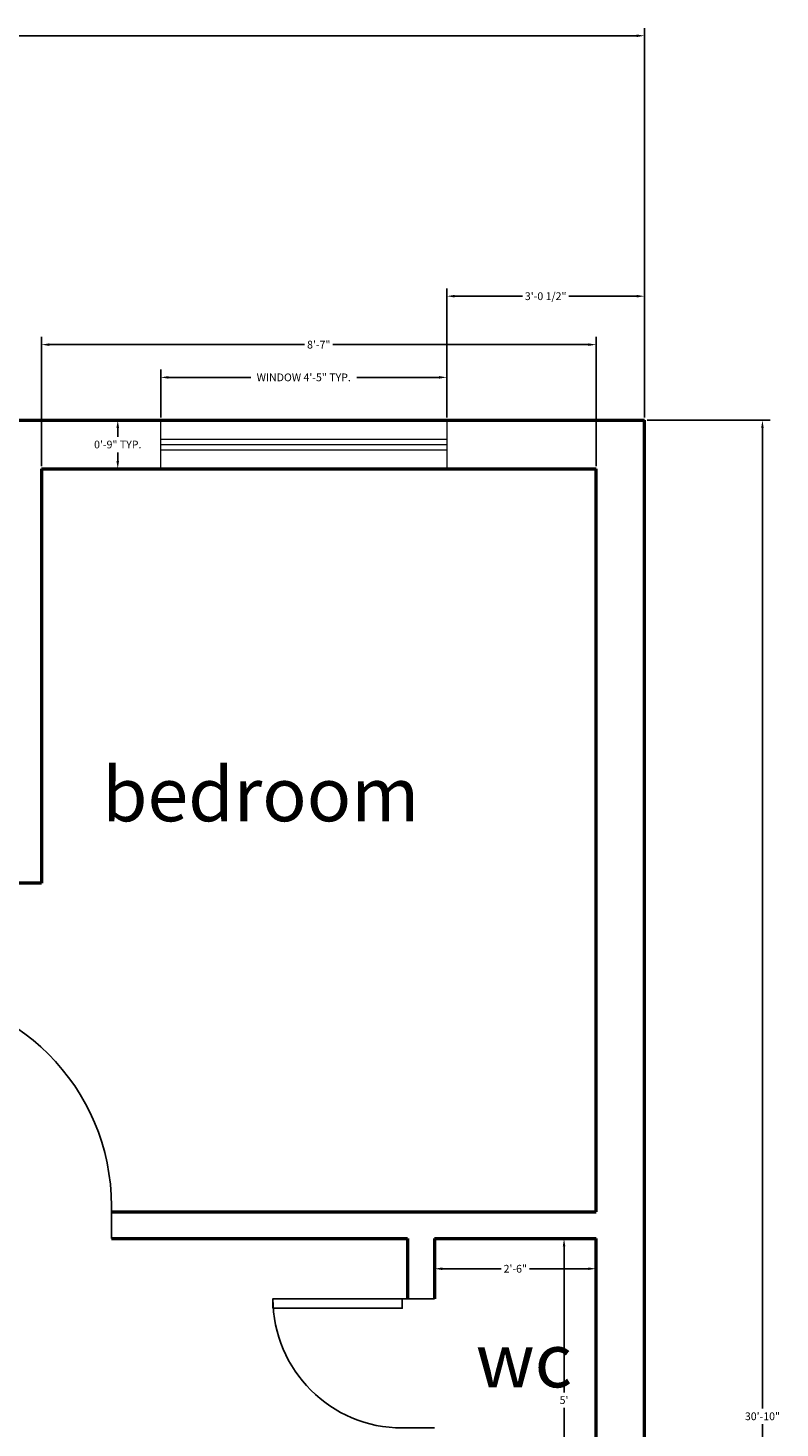
# Model space of a CAD drawing. Units: inches. Extents: x 325 to 804, y 366 to 834.
# Tile 6 of 6: x 660 to 800, y 574 to 834. Entities that reach past the tile are written whole.
import ezdxf

# ---------------------------------------------------------------- set-up
doc = ezdxf.new("R2010")
doc.units = ezdxf.units.IN
doc.header["$MEASUREMENT"] = 0
doc.layers.get('0').update_dxf_attribs({"color": 4})
for name, color, linetype, lineweight in [('A-ANNO-DIMS', 2, 'Continuous', 18), ('A-AREA-IDEN', 7, 'Continuous', 25), ('A-WALL', 7, 'Continuous', 50), ('door', 10, 'Continuous', 25), ('window', 3, 'Continuous', 18)]:
    doc.layers.add(name, color=color, linetype=linetype, lineweight=lineweight)
doc.styles.get("Standard").update_dxf_attribs({"font": 'arial.ttf'})
doc.dimstyles.get("Standard").update_dxf_attribs({"dimscale": 8, "dimtxt": 0.18, "dimasz": 0.18, "dimexe": 0.18, "dimexo": 0.0625, "dimgap": 0.09, "dimtad": 0, "dimtih": 1, "dimtoh": 1, "dimdec": 0, "dimzin": 0, "dimdsep": 46, "dimlunit": 3, "dimtxsty": 'Standard', "dimcen": 0.09, "dimadec": 0, "dimazin": 0, "dimtfac": 1, "dimtdec": 0, "dimtofl": 0, "dimtmove": 0, "dimatfit": 3, "dimfxl": 1, "dimtolj": 1, "dimtzin": 0, "dimarcsym": 0})

# ---------------------------------------------------------------- blocks, each defined once
blk = doc.blocks.new('*U2')
for p, q in [((0, 0), (0, -6)), ((-40, 0), (-40, -6))]:
    blk.add_line(p, q)
blk.add_lwpolyline([(0, 0), (0, 40), (-1.75, 40), (-1.75, 0)], close=True)
blk.add_arc((0, 0), 40, 90, 180)
blk = doc.blocks.new('*U8')
for p, q in [((-24, 0), (-24, -6)), ((0, 0), (0, -6))]:
    blk.add_line(p, q)
blk.add_lwpolyline([(0, 0), (0, 24), (-1.75, 24), (-1.75, 0)], close=True)
blk.add_arc((0, 0), 24, 90, 180)
blk = doc.blocks.new('*D21')
at = {"layer": 'A-ANNO-DIMS', "color": 0, "lineweight": -2, "transparency": 16777216}
for p, q in [((764.97, 609.54), (758.08, 609.54)), ((759.52, 608.1), (759.52, 580.99)), ((759.52, 550.98), (759.52, 578.09)), ((764.97, 549.54), (758.08, 549.54))]:
    blk.add_line(p, q, dxfattribs=at)
at = {"layer": 'A-ANNO-DIMS', "color": 0, "transparency": 16777216}
for points in [[(759.28, 608.1), (759.76, 608.1), (759.52, 609.54)], [(759.28, 550.98), (759.76, 550.98), (759.52, 549.54)]]:
    blk.add_solid(points, dxfattribs=at)
at = {"layer": 'Defpoints', "color": 0, "transparency": 16777216}
for p in [(765.47, 609.54), (759.52, 549.54), (765.47, 549.54)]:
    blk.add_point(p, dxfattribs=at)
at = {"layer": 'A-ANNO-DIMS', "color": 0, "transparency": 16777216, "insert": (759.52, 579.54), "char_height": 1.44, "attachment_point": 5}
blk.add_mtext("\\A1;5'", dxfattribs=at)
blk = doc.blocks.new('*D22')
at = {"layer": 'A-ANNO-DIMS', "color": 0, "lineweight": -2, "transparency": 16777216}
for p, q in [((735.47, 609.04), (735.47, 602.51)), ((765.47, 609.04), (765.47, 602.51)), ((736.91, 603.95), (747.83, 603.95)), ((764.03, 603.95), (753.12, 603.95))]:
    blk.add_line(p, q, dxfattribs=at)
at = {"layer": 'A-ANNO-DIMS', "color": 0, "transparency": 16777216}
for points in [[(736.91, 604.19), (736.91, 603.71), (735.47, 603.95)], [(764.03, 604.19), (764.03, 603.71), (765.47, 603.95)]]:
    blk.add_solid(points, dxfattribs=at)
at = {"layer": 'Defpoints', "color": 0, "transparency": 16777216}
for p in [(735.47, 609.54), (765.47, 609.54), (735.47, 603.95)]:
    blk.add_point(p, dxfattribs=at)
at = {"layer": 'A-ANNO-DIMS', "color": 0, "transparency": 16777216, "insert": (750.47, 603.95), "char_height": 1.44, "attachment_point": 5}
blk.add_mtext('\\A1;2\'-6"', dxfattribs=at)
blk = doc.blocks.new('*D25')
at = {"layer": 'A-ANNO-DIMS', "color": 0, "lineweight": -2, "transparency": 16777216}
for p, q in [((350.47, 762.04), (350.47, 834.4)), ((351.91, 832.96), (559.28, 832.96)), ((773.03, 832.96), (565.67, 832.96)), ((774.47, 762.04), (774.47, 834.4))]:
    blk.add_line(p, q, dxfattribs=at)
at = {"layer": 'A-ANNO-DIMS', "color": 0, "transparency": 16777216}
for points in [[(351.91, 833.2), (351.91, 832.72), (350.47, 832.96)], [(773.03, 833.2), (773.03, 832.72), (774.47, 832.96)]]:
    blk.add_solid(points, dxfattribs=at)
at = {"layer": 'Defpoints', "color": 0, "transparency": 16777216}
for p in [(774.47, 832.96), (350.47, 761.54), (774.47, 761.54)]:
    blk.add_point(p, dxfattribs=at)
at = {"layer": 'A-ANNO-DIMS', "color": 0, "transparency": 16777216, "insert": (562.47, 832.96), "char_height": 1.44, "attachment_point": 5}
blk.add_mtext('\\A1;35\'-4"', dxfattribs=at)
blk = doc.blocks.new('*D26')
at = {"layer": 'A-ANNO-DIMS', "color": 0, "lineweight": -2, "transparency": 16777216}
for p, q in [((774.97, 761.54), (797.81, 761.54)), ((796.37, 760.1), (796.37, 577.99)), ((796.37, 392.98), (796.37, 575.08)), ((774.97, 391.54), (797.81, 391.54))]:
    blk.add_line(p, q, dxfattribs=at)
at = {"layer": 'A-ANNO-DIMS', "color": 0, "transparency": 16777216}
for points in [[(796.13, 760.1), (796.61, 760.1), (796.37, 761.54)], [(796.13, 392.98), (796.61, 392.98), (796.37, 391.54)]]:
    blk.add_solid(points, dxfattribs=at)
at = {"layer": 'Defpoints', "color": 0, "transparency": 16777216}
for p in [(774.47, 761.54), (774.47, 391.54), (796.37, 391.54)]:
    blk.add_point(p, dxfattribs=at)
at = {"layer": 'A-ANNO-DIMS', "color": 0, "transparency": 16777216, "insert": (796.37, 576.54), "char_height": 1.44, "attachment_point": 5}
blk.add_mtext('\\A1;30\'-10"', dxfattribs=at)
blk = doc.blocks.new('WIN-53_14x9')
for p, q in [((0, 5.5), (53.14, 5.5)), ((0, 4.5), (53.14, 4.5)), ((0, 3.5), (53.14, 3.5))]:
    blk.add_line(p, q)
blk.add_lwpolyline([(0, 9), (53.14, 9), (53.14, 0), (0, 0)], close=True)
blk = doc.blocks.new('*D28')
at = {"layer": 'A-ANNO-DIMS', "color": 0, "lineweight": -2, "transparency": 16777216}
for p, q in [((684.61, 762.04), (684.61, 770.95)), ((737.75, 762.04), (737.75, 770.95)), ((686.05, 769.51), (701.35, 769.51)), ((736.31, 769.51), (721.01, 769.51))]:
    blk.add_line(p, q, dxfattribs=at)
at = {"layer": 'A-ANNO-DIMS', "color": 0, "transparency": 16777216}
for points in [[(686.05, 769.75), (686.05, 769.27), (684.61, 769.51)], [(736.31, 769.75), (736.31, 769.27), (737.75, 769.51)]]:
    blk.add_solid(points, dxfattribs=at)
at = {"layer": 'Defpoints', "color": 0, "transparency": 16777216}
for p in [(737.75, 769.51), (684.61, 761.54), (737.75, 761.54)]:
    blk.add_point(p, dxfattribs=at)
at = {"layer": 'A-ANNO-DIMS', "color": 0, "transparency": 16777216, "insert": (711.18, 769.51), "char_height": 1.44, "attachment_point": 5}
blk.add_mtext('\\A1;WINDOW 4\'-5" TYP.', dxfattribs=at)
blk = doc.blocks.new('*D29')
at = {"layer": 'A-ANNO-DIMS', "color": 0, "lineweight": -2, "transparency": 16777216}
for p, q in [((684.11, 761.54), (675.2, 761.54)), ((676.64, 760.1), (676.64, 758.49)), ((676.64, 753.98), (676.64, 755.58)), ((684.11, 752.54), (675.2, 752.54))]:
    blk.add_line(p, q, dxfattribs=at)
at = {"layer": 'A-ANNO-DIMS', "color": 0, "transparency": 16777216}
for points in [[(676.4, 760.1), (676.88, 760.1), (676.64, 761.54)], [(676.4, 753.98), (676.88, 753.98), (676.64, 752.54)]]:
    blk.add_solid(points, dxfattribs=at)
at = {"layer": 'Defpoints', "color": 0, "transparency": 16777216}
for p in [(676.64, 761.54), (684.61, 761.54), (684.61, 752.54)]:
    blk.add_point(p, dxfattribs=at)
at = {"layer": 'A-ANNO-DIMS', "color": 0, "transparency": 16777216, "insert": (676.64, 757.04), "char_height": 1.44, "attachment_point": 5}
blk.add_mtext('\\A1;0\'-9" TYP.', dxfattribs=at)
blk = doc.blocks.new('*D32')
at = {"layer": 'A-ANNO-DIMS', "color": 0, "lineweight": -2, "transparency": 16777216}
for p, q in [((737.75, 762.04), (737.75, 786.03)), ((774.47, 762.04), (774.47, 786.03)), ((739.19, 784.59), (751.8, 784.59)), ((773.03, 784.59), (760.42, 784.59))]:
    blk.add_line(p, q, dxfattribs=at)
at = {"layer": 'A-ANNO-DIMS', "color": 0, "transparency": 16777216}
for points in [[(739.19, 784.83), (739.19, 784.35), (737.75, 784.59)], [(773.03, 784.83), (773.03, 784.35), (774.47, 784.59)]]:
    blk.add_solid(points, dxfattribs=at)
at = {"layer": 'Defpoints', "color": 0, "transparency": 16777216}
for p in [(774.47, 784.59), (737.75, 761.54), (774.47, 761.54)]:
    blk.add_point(p, dxfattribs=at)
at = {"layer": 'A-ANNO-DIMS', "color": 0, "transparency": 16777216, "insert": (756.11, 784.59), "char_height": 1.44, "attachment_point": 5}
blk.add_mtext('\\A1;3\'-0 1/2"', dxfattribs=at)
blk = doc.blocks.new('*D35')
at = {"layer": 'A-ANNO-DIMS', "color": 0, "lineweight": -2, "transparency": 16777216}
for p, q in [((662.47, 753.04), (662.47, 777.03)), ((663.91, 775.59), (711.34, 775.59)), ((764.03, 775.59), (716.61, 775.59)), ((765.47, 753.04), (765.47, 777.03))]:
    blk.add_line(p, q, dxfattribs=at)
at = {"layer": 'A-ANNO-DIMS', "color": 0, "transparency": 16777216}
for points in [[(663.91, 775.83), (663.91, 775.35), (662.47, 775.59)], [(764.03, 775.83), (764.03, 775.35), (765.47, 775.59)]]:
    blk.add_solid(points, dxfattribs=at)
at = {"layer": 'Defpoints', "color": 0, "transparency": 16777216}
for p in [(765.47, 775.59), (662.47, 752.54), (765.47, 752.54)]:
    blk.add_point(p, dxfattribs=at)
at = {"layer": 'A-ANNO-DIMS', "color": 0, "transparency": 16777216, "insert": (713.97, 775.59), "char_height": 1.44, "attachment_point": 5}
blk.add_mtext('\\A1;8\'-7"', dxfattribs=at)

msp = doc.modelspace()

# ---------------------------------------------------------------- linework, layer by layer
at = {"layer": 'A-WALL'}
for p, q in [((350.47, 761.54), (774.47, 761.54)), ((774.47, 391.54), (774.47, 761.54)), ((662.47, 752.54), (662.47, 675.54)), ((662.47, 752.54), (765.47, 752.54)), ((765.47, 614.54), (765.47, 752.54)), ((662.47, 675.54), (633.47, 675.54)), ((675.47, 614.54), (765.47, 614.54)), ((675.47, 609.54), (730.47, 609.54)), ((730.47, 609.54), (730.47, 598.37)), ((735.47, 609.54), (735.47, 598.37)), ((735.47, 609.54), (765.47, 609.54)), ((765.47, 549.54), (765.47, 609.54))]:
    msp.add_line(p, q, dxfattribs=at)
at = {"layer": 'door'}
msp.add_line((735.47, 598.37), (730.47, 598.37), dxfattribs=at)

# ---------------------------------------------------------------- block references
at = {"layer": 'door', "xscale": -1}
msp.add_blockref('*U2', (635.47, 615.54), dxfattribs=at)
at = {"layer": 'door', "rotation": 90}
msp.add_blockref('*U8', (729.47, 598.37), dxfattribs=at)
at = {"layer": 'window'}
msp.add_blockref('WIN-53_14x9', (684.61, 752.54), dxfattribs=at)

# ---------------------------------------------------------------- texts
at = {"layer": 'A-AREA-IDEN', "char_height": 10, "attachment_point": 1}
for s, width, insert in [('bedroom', 79.8504, (673.73, 697.06)), ('wc', 25.6907, (743.12, 591.93))]:
    msp.add_mtext_dynamic_manual_height_columns(s, width=width, gutter_width=1, heights=[0], dxfattribs=dict(at, insert=insert))

# ---------------------------------------------------------------- dimensions: what is measured, and where the dimension line sits
at = {"layer": 'A-ANNO-DIMS'}
for base, p1, p2, override, picture, middle in [((774.47, 832.96), (350.47, 761.54), (774.47, 761.54), {"dimclrd": 0, "dimclre": 0, "dimclrt": 0}, '*D25', (562.47, 832.96)), ((774.47, 784.59), (737.75, 761.54), (774.47, 761.54), {"dimdec": 1, "dimlfac": 1, "dimrnd": 0, "dimzin": 1, "dimdsep": 46, "dimlunit": 4, "dimfrac": 2}, '*D32', (756.11, 784.59)), ((765.47, 775.59), (662.47, 752.54), (765.47, 752.54), {"dimdec": 1, "dimlfac": 1, "dimrnd": 0, "dimzin": 1, "dimdsep": 46, "dimlunit": 4, "dimfrac": 2}, '*D35', (713.97, 775.59)), ((735.47, 603.95), (765.47, 609.54), (735.47, 609.54), {"dimclrd": 0, "dimclre": 0, "dimclrt": 0}, '*D22', (750.47, 603.95))]:
    dim = msp.add_linear_dim(base=base, p1=p1, p2=p2, dimstyle='Standard', override=override, dxfattribs=at)
    dim.commit()
    dim.dimension.update_dxf_attribs({"geometry": picture, "text_midpoint": middle})
dim = msp.add_linear_dim(base=(737.75, 769.51), p1=(684.61, 761.54), p2=(737.75, 761.54), text='WINDOW <> TYP.', dimstyle='Standard', override={"dimdec": 1, "dimlfac": 1, "dimrnd": 0, "dimzin": 1, "dimdsep": 46, "dimlunit": 4, "dimfrac": 2}, dxfattribs=at)
dim.commit()
dim.dimension.update_dxf_attribs({"geometry": '*D28', "text_midpoint": (711.18, 769.51)})
dim = msp.add_linear_dim(base=(676.64, 761.54), p1=(684.61, 752.54), p2=(684.61, 761.54), angle=90, text='<> TYP.', dimstyle='Standard', override={"dimdec": 1, "dimlfac": 1, "dimrnd": 0, "dimzin": 1, "dimdsep": 46, "dimlunit": 4, "dimfrac": 2}, dxfattribs=at)
dim.commit()
dim.dimension.update_dxf_attribs({"geometry": '*D29', "text_midpoint": (676.64, 757.04)})
for base, p1, p2, picture, middle in [((796.37, 391.54), (774.47, 761.54), (774.47, 391.54), '*D26', (796.37, 576.54)), ((759.52, 549.54), (765.47, 609.54), (765.47, 549.54), '*D21', (759.52, 579.54))]:
    dim = msp.add_linear_dim(base=base, p1=p1, p2=p2, angle=90, dimstyle='Standard', override={"dimclrd": 0, "dimclre": 0, "dimclrt": 0}, dxfattribs=at)
    dim.commit()
    dim.dimension.update_dxf_attribs({"geometry": picture, "text_midpoint": middle})

doc.saveas('drawing.dxf')
